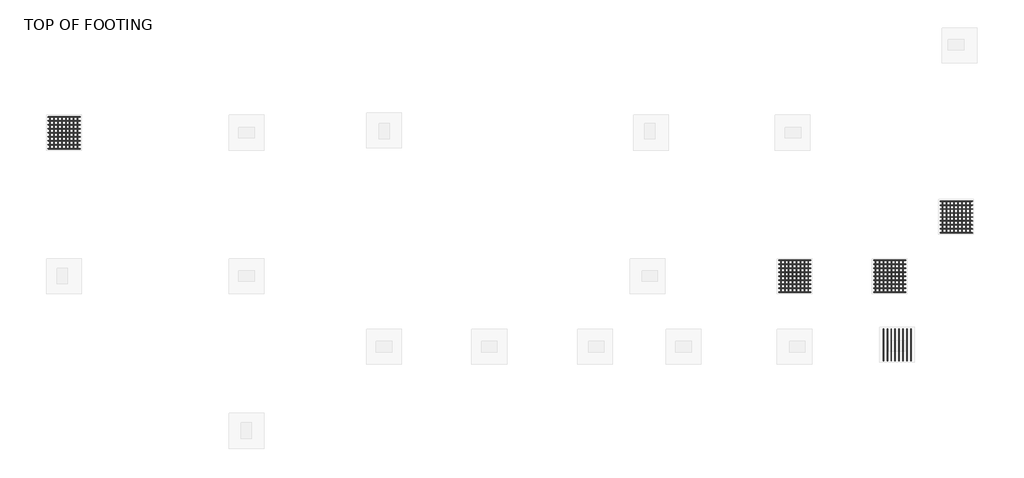
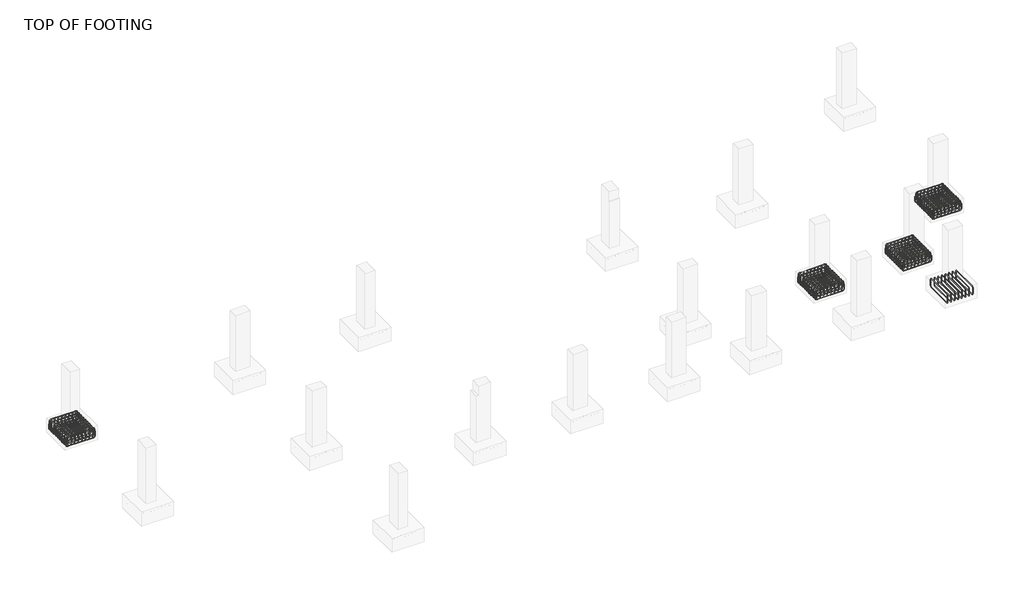
# One storey, part 10 of 20: 18 reinforcing bars.
"""IFC4 building model written with IfcOpenShell, lengths in millimetres."""

from ifc_helpers import new_model, si_unit, point, frame, origin, place, context, project, spatial, polyline, circle_curve, trimmed, segment, composite_curve, source, transform, mapped, element, save
from ifc_brep_helpers import swept_disk

model = new_model("IFC4")

# Units and contexts
model_context = context("Model", 3, world=origin())
ifc_project = project(units=[si_unit("LENGTHUNIT", "METRE", prefix="MILLI")], contexts=[model_context])

# Site, building, storey
site = spatial("IfcSite", under=ifc_project)
building = spatial("IfcBuilding", under=site)
storey = spatial("IfcBuildingStorey", under=building, Name="TOP OF FOOTING", Elevation=-1828.8)

# Reinforcing bars
placement = place(None, origin())
reinforcing_bar_shape = source(origin(), model_context, "Body", "SolidModel", [
    swept_disk(composite_curve([segment(polyline([(14922.7663908, -845.1786071, -2006.6587682), (14922.7663908, -845.1786071, -2153.9587682)]), True, "CONTINUOUS"), segment(trimmed(circle_curve(frame((14876.4163908, -845.1786071, -2153.9587682), z_axis=(0.0, 1.0, 0.0), x_axis=(46.350000000000364, 0.0, 0.0)), 46.35), [point((14922.7663908, -845.1786071, -2153.9587682))], [point((14876.4163908, -845.1786071, -2200.3087682))], True, "CARTESIAN"), True, "CONTINUOUS"), segment(polyline([(14876.4163908, -845.1786071, -2200.3087682), (14061.8163908, -845.1786071, -2200.3087682)]), True, "CONTINUOUS"), segment(trimmed(circle_curve(frame((14061.8163908, -845.1786071, -2153.9587682), z_axis=(0.0, 1.0, 0.0), x_axis=(0.0, 0.0, -46.34999999999991)), 46.35), [point((14061.8163908, -845.1786071, -2200.3087682))], [point((14015.4663908, -845.1786071, -2153.9587682))], True, "CARTESIAN"), True, "CONTINUOUS"), segment(polyline([(14015.4663908, -845.1786071, -2153.9587682), (14015.4663908, -845.1786071, -2006.6587682)]), True, "CONTINUOUS")], self_intersect=False), 6.35),
])
element("IfcReinforcingBar", 1, at=placement, inside=storey, context=model_context, shape_type="MappedRepresentation", body=[
    mapped(reinforcing_bar_shape, transform((0.0, 0.0, 0.0), x_axis=(1.0, 0.0, 0.0), y_axis=(0.0, 1.0, 0.0), z_axis=(0.0, 0.0, 1.0))),
    mapped(reinforcing_bar_shape, transform((0.0, -113.4125, 0.0), x_axis=(1.0, 0.0, 0.0), y_axis=(0.0, 1.0, 0.0), z_axis=(0.0, 0.0, 1.0))),
    mapped(reinforcing_bar_shape, transform((0.0, -226.825, 0.0), x_axis=(1.0, 0.0, 0.0), y_axis=(0.0, 1.0, 0.0), z_axis=(0.0, 0.0, 1.0))),
    mapped(reinforcing_bar_shape, transform((0.0, -340.2375, 0.0), x_axis=(1.0, 0.0, 0.0), y_axis=(0.0, 1.0, 0.0), z_axis=(0.0, 0.0, 1.0))),
    mapped(reinforcing_bar_shape, transform((0.0, -453.65, 0.0), x_axis=(1.0, 0.0, 0.0), y_axis=(0.0, 1.0, 0.0), z_axis=(0.0, 0.0, 1.0))),
    mapped(reinforcing_bar_shape, transform((0.0, -567.0625, 0.0), x_axis=(1.0, 0.0, 0.0), y_axis=(0.0, 1.0, 0.0), z_axis=(0.0, 0.0, 1.0))),
    mapped(reinforcing_bar_shape, transform((0.0, -680.475, 0.0), x_axis=(1.0, 0.0, 0.0), y_axis=(0.0, 1.0, 0.0), z_axis=(0.0, 0.0, 1.0))),
    mapped(reinforcing_bar_shape, transform((0.0, -793.8875, 0.0), x_axis=(1.0, 0.0, 0.0), y_axis=(0.0, 1.0, 0.0), z_axis=(0.0, 0.0, 1.0))),
    mapped(reinforcing_bar_shape, transform((0.0, -907.3, 0.0), x_axis=(1.0, 0.0, 0.0), y_axis=(0.0, 1.0, 0.0), z_axis=(0.0, 0.0, 1.0))),
])
reinforcing_bar_2_shape = source(origin(), model_context, "Body", "SolidModel", [
    swept_disk(composite_curve([segment(polyline([(14034.9405021, -845.1786071, -2068.8), (14034.9405021, -845.1786071, -1921.5)]), True, "CONTINUOUS"), segment(trimmed(circle_curve(frame((14081.2905021, -845.1786071, -1921.5), z_axis=(0.0, 1.0, 0.0), x_axis=(-46.350000000000364, 0.0, 0.0)), 46.35), [point((14034.9405021, -845.1786071, -1921.5))], [point((14081.2905021, -845.1786071, -1875.15))], True, "CARTESIAN"), True, "CONTINUOUS"), segment(polyline([(14081.2905021, -845.1786071, -1875.15), (14850.7539017, -845.1786071, -1875.15)]), True, "CONTINUOUS"), segment(trimmed(circle_curve(frame((14850.7539017, -845.1786071, -1921.5), z_axis=(0.0, 1.0, 0.0), x_axis=(0.0, 0.0, 46.34999999999991)), 46.35), [point((14850.7539017, -845.1786071, -1875.15))], [point((14897.1039017, -845.1786071, -1921.5))], True, "CARTESIAN"), True, "CONTINUOUS"), segment(polyline([(14897.1039017, -845.1786071, -1921.5), (14897.1039017, -845.1786071, -2068.8)]), True, "CONTINUOUS")], self_intersect=False), 6.35),
])
element("IfcReinforcingBar", 2, at=placement, inside=storey, context=model_context, shape_type="MappedRepresentation", body=[
    mapped(reinforcing_bar_2_shape, transform((0.0, 0.0, 0.0), x_axis=(1.0, 0.0, 0.0), y_axis=(0.0, 1.0, 0.0), z_axis=(0.0, 0.0, 1.0))),
    mapped(reinforcing_bar_2_shape, transform((0.0, -113.4125, 0.0), x_axis=(1.0, 0.0, 0.0), y_axis=(0.0, 1.0, 0.0), z_axis=(0.0, 0.0, 1.0))),
    mapped(reinforcing_bar_2_shape, transform((0.0, -226.825, 0.0), x_axis=(1.0, 0.0, 0.0), y_axis=(0.0, 1.0, 0.0), z_axis=(0.0, 0.0, 1.0))),
    mapped(reinforcing_bar_2_shape, transform((0.0, -340.2375, 0.0), x_axis=(1.0, 0.0, 0.0), y_axis=(0.0, 1.0, 0.0), z_axis=(0.0, 0.0, 1.0))),
    mapped(reinforcing_bar_2_shape, transform((0.0, -453.65, 0.0), x_axis=(1.0, 0.0, 0.0), y_axis=(0.0, 1.0, 0.0), z_axis=(0.0, 0.0, 1.0))),
    mapped(reinforcing_bar_2_shape, transform((0.0, -567.0625, 0.0), x_axis=(1.0, 0.0, 0.0), y_axis=(0.0, 1.0, 0.0), z_axis=(0.0, 0.0, 1.0))),
    mapped(reinforcing_bar_2_shape, transform((0.0, -680.475, 0.0), x_axis=(1.0, 0.0, 0.0), y_axis=(0.0, 1.0, 0.0), z_axis=(0.0, 0.0, 1.0))),
    mapped(reinforcing_bar_2_shape, transform((0.0, -793.8875, 0.0), x_axis=(1.0, 0.0, 0.0), y_axis=(0.0, 1.0, 0.0), z_axis=(0.0, 0.0, 1.0))),
    mapped(reinforcing_bar_2_shape, transform((0.0, -907.3, 0.0), x_axis=(1.0, 0.0, 0.0), y_axis=(0.0, 1.0, 0.0), z_axis=(0.0, 0.0, 1.0))),
])
reinforcing_bar_3_shape = source(origin(), model_context, "Body", "SolidModel", [
    swept_disk(composite_curve([segment(polyline([(14851.2694294, -845.1786071, -2086.1951968), (14851.2694294, -845.1786071, -1938.8951968)]), True, "CONTINUOUS"), segment(trimmed(circle_curve(frame((14851.2694294, -891.5286071, -1938.8951968), z_axis=(1.0, 0.0, 0.0), x_axis=(0.0, 46.35000000000002, 0.0)), 46.35), [point((14851.2694294, -845.1786071, -1938.8951968))], [point((14851.2694294, -891.5286071, -1892.5451968))], True, "CARTESIAN"), True, "CONTINUOUS"), segment(polyline([(14851.2694294, -891.5286071, -1892.5451968), (14851.2694294, -1706.1286071, -1892.5451968)]), True, "CONTINUOUS"), segment(trimmed(circle_curve(frame((14851.2694294, -1706.1286071, -1938.8951968), z_axis=(1.0, 0.0, 0.0), x_axis=(0.0, 0.0, 46.34999999999991)), 46.35), [point((14851.2694294, -1706.1286071, -1892.5451968))], [point((14851.2694294, -1752.4786071, -1938.8951968))], True, "CARTESIAN"), True, "CONTINUOUS"), segment(polyline([(14851.2694294, -1752.4786071, -1938.8951968), (14851.2694294, -1752.4786071, -2086.1951968)]), True, "CONTINUOUS")], self_intersect=False), 6.35),
])
element("IfcReinforcingBar", 3, at=placement, inside=storey, context=model_context, shape_type="MappedRepresentation", body=[
    mapped(reinforcing_bar_3_shape, transform((0.0, 0.0, 0.0), x_axis=(1.0, 0.0, 0.0), y_axis=(0.0, 1.0, 0.0), z_axis=(0.0, 0.0, 1.0))),
    mapped(reinforcing_bar_3_shape, transform((-111.2862402, 0.0, 0.0), x_axis=(1.0, 0.0, 0.0), y_axis=(0.0, 1.0, 0.0), z_axis=(0.0, 0.0, 1.0))),
    mapped(reinforcing_bar_3_shape, transform((-222.5724804, 0.0, 0.0), x_axis=(1.0, 0.0, 0.0), y_axis=(0.0, 1.0, 0.0), z_axis=(0.0, 0.0, 1.0))),
    mapped(reinforcing_bar_3_shape, transform((-333.8587205, 0.0, 0.0), x_axis=(1.0, 0.0, 0.0), y_axis=(0.0, 1.0, 0.0), z_axis=(0.0, 0.0, 1.0))),
    mapped(reinforcing_bar_3_shape, transform((-445.1449607, 0.0, 0.0), x_axis=(1.0, 0.0, 0.0), y_axis=(0.0, 1.0, 0.0), z_axis=(0.0, 0.0, 1.0))),
    mapped(reinforcing_bar_3_shape, transform((-556.4312009, 0.0, 0.0), x_axis=(1.0, 0.0, 0.0), y_axis=(0.0, 1.0, 0.0), z_axis=(0.0, 0.0, 1.0))),
    mapped(reinforcing_bar_3_shape, transform((-667.7174411, 0.0, 0.0), x_axis=(1.0, 0.0, 0.0), y_axis=(0.0, 1.0, 0.0), z_axis=(0.0, 0.0, 1.0))),
    mapped(reinforcing_bar_3_shape, transform((-779.0036813, 0.0, 0.0), x_axis=(1.0, 0.0, 0.0), y_axis=(0.0, 1.0, 0.0), z_axis=(0.0, 0.0, 1.0))),
])
reinforcing_bar_4_shape = source(origin(), model_context, "Body", "SolidModel", [
    swept_disk(composite_curve([segment(polyline([(14072.2657481, -845.1786071, -1979.1645013), (14072.2657481, -845.1786071, -2126.4645013)]), True, "CONTINUOUS"), segment(trimmed(circle_curve(frame((14072.2657481, -891.5286071, -2126.4645013), z_axis=(-1.0, 0.0, 0.0), x_axis=(0.0, 46.35000000000002, 0.0)), 46.35), [point((14072.2657481, -845.1786071, -2126.4645013))], [point((14072.2657481, -891.5286071, -2172.8145013))], True, "CARTESIAN"), True, "CONTINUOUS"), segment(polyline([(14072.2657481, -891.5286071, -2172.8145013), (14072.2657481, -1706.1286071, -2172.8145013)]), True, "CONTINUOUS"), segment(trimmed(circle_curve(frame((14072.2657481, -1706.1286071, -2126.4645013), z_axis=(-1.0, 0.0, 0.0), x_axis=(0.0, 0.0, -46.34999999999991)), 46.35), [point((14072.2657481, -1706.1286071, -2172.8145013))], [point((14072.2657481, -1752.4786071, -2126.4645013))], True, "CARTESIAN"), True, "CONTINUOUS"), segment(polyline([(14072.2657481, -1752.4786071, -2126.4645013), (14072.2657481, -1752.4786071, -1979.1645013)]), True, "CONTINUOUS")], self_intersect=False), 6.35),
])
element("IfcReinforcingBar", 4, at=placement, inside=storey, context=model_context, shape_type="MappedRepresentation", body=[
    mapped(reinforcing_bar_4_shape, transform((0.0, 0.0, 0.0), x_axis=(1.0, 0.0, 0.0), y_axis=(0.0, 1.0, 0.0), z_axis=(0.0, 0.0, 1.0))),
    mapped(reinforcing_bar_4_shape, transform((111.2862402, 0.0, 0.0), x_axis=(1.0, 0.0, 0.0), y_axis=(0.0, 1.0, 0.0), z_axis=(0.0, 0.0, 1.0))),
    mapped(reinforcing_bar_4_shape, transform((222.5724804, 0.0, 0.0), x_axis=(1.0, 0.0, 0.0), y_axis=(0.0, 1.0, 0.0), z_axis=(0.0, 0.0, 1.0))),
    mapped(reinforcing_bar_4_shape, transform((333.8587205, 0.0, 0.0), x_axis=(1.0, 0.0, 0.0), y_axis=(0.0, 1.0, 0.0), z_axis=(0.0, 0.0, 1.0))),
    mapped(reinforcing_bar_4_shape, transform((445.1449607, 0.0, 0.0), x_axis=(1.0, 0.0, 0.0), y_axis=(0.0, 1.0, 0.0), z_axis=(0.0, 0.0, 1.0))),
    mapped(reinforcing_bar_4_shape, transform((556.4312009, 0.0, 0.0), x_axis=(1.0, 0.0, 0.0), y_axis=(0.0, 1.0, 0.0), z_axis=(0.0, 0.0, 1.0))),
    mapped(reinforcing_bar_4_shape, transform((667.7174411, 0.0, 0.0), x_axis=(1.0, 0.0, 0.0), y_axis=(0.0, 1.0, 0.0), z_axis=(0.0, 0.0, 1.0))),
    mapped(reinforcing_bar_4_shape, transform((779.0036813, 0.0, 0.0), x_axis=(1.0, 0.0, 0.0), y_axis=(0.0, 1.0, 0.0), z_axis=(0.0, 0.0, 1.0))),
])
reinforcing_bar_5_shape = source(origin(), model_context, "Body", "SolidModel", [
    swept_disk(composite_curve([segment(polyline([(13022.7663908, -2535.8035766, -2006.6587682), (13022.7663908, -2535.8035766, -2153.9587682)]), True, "CONTINUOUS"), segment(trimmed(circle_curve(frame((12976.4163908, -2535.8035766, -2153.9587682), z_axis=(0.0, 1.0, 0.0), x_axis=(46.350000000000364, 0.0, 0.0)), 46.35), [point((13022.7663908, -2535.8035766, -2153.9587682))], [point((12976.4163908, -2535.8035766, -2200.3087682))], True, "CARTESIAN"), True, "CONTINUOUS"), segment(polyline([(12976.4163908, -2535.8035766, -2200.3087682), (12161.8163908, -2535.8035766, -2200.3087682)]), True, "CONTINUOUS"), segment(trimmed(circle_curve(frame((12161.8163908, -2535.8035766, -2153.9587682), z_axis=(0.0, 1.0, 0.0), x_axis=(0.0, 0.0, -46.34999999999991)), 46.35), [point((12161.8163908, -2535.8035766, -2200.3087682))], [point((12115.4663908, -2535.8035766, -2153.9587682))], True, "CARTESIAN"), True, "CONTINUOUS"), segment(polyline([(12115.4663908, -2535.8035766, -2153.9587682), (12115.4663908, -2535.8035766, -2006.6587682)]), True, "CONTINUOUS")], self_intersect=False), 6.35),
])
element("IfcReinforcingBar", 5, at=placement, inside=storey, context=model_context, shape_type="MappedRepresentation", body=[
    mapped(reinforcing_bar_5_shape, transform((0.0, 0.0, 0.0), x_axis=(1.0, 0.0, 0.0), y_axis=(0.0, 1.0, 0.0), z_axis=(0.0, 0.0, 1.0))),
    mapped(reinforcing_bar_5_shape, transform((0.0, -113.4125, 0.0), x_axis=(1.0, 0.0, 0.0), y_axis=(0.0, 1.0, 0.0), z_axis=(0.0, 0.0, 1.0))),
    mapped(reinforcing_bar_5_shape, transform((0.0, -226.825, 0.0), x_axis=(1.0, 0.0, 0.0), y_axis=(0.0, 1.0, 0.0), z_axis=(0.0, 0.0, 1.0))),
    mapped(reinforcing_bar_5_shape, transform((0.0, -340.2375, 0.0), x_axis=(1.0, 0.0, 0.0), y_axis=(0.0, 1.0, 0.0), z_axis=(0.0, 0.0, 1.0))),
    mapped(reinforcing_bar_5_shape, transform((0.0, -453.65, 0.0), x_axis=(1.0, 0.0, 0.0), y_axis=(0.0, 1.0, 0.0), z_axis=(0.0, 0.0, 1.0))),
    mapped(reinforcing_bar_5_shape, transform((0.0, -567.0625, 0.0), x_axis=(1.0, 0.0, 0.0), y_axis=(0.0, 1.0, 0.0), z_axis=(0.0, 0.0, 1.0))),
    mapped(reinforcing_bar_5_shape, transform((0.0, -680.475, 0.0), x_axis=(1.0, 0.0, 0.0), y_axis=(0.0, 1.0, 0.0), z_axis=(0.0, 0.0, 1.0))),
    mapped(reinforcing_bar_5_shape, transform((0.0, -793.8875, 0.0), x_axis=(1.0, 0.0, 0.0), y_axis=(0.0, 1.0, 0.0), z_axis=(0.0, 0.0, 1.0))),
    mapped(reinforcing_bar_5_shape, transform((0.0, -907.3, 0.0), x_axis=(1.0, 0.0, 0.0), y_axis=(0.0, 1.0, 0.0), z_axis=(0.0, 0.0, 1.0))),
])
reinforcing_bar_6_shape = source(origin(), model_context, "Body", "SolidModel", [
    swept_disk(composite_curve([segment(polyline([(12134.9405021, -2535.8035766, -2068.8), (12134.9405021, -2535.8035766, -1921.5)]), True, "CONTINUOUS"), segment(trimmed(circle_curve(frame((12181.2905021, -2535.8035766, -1921.5), z_axis=(0.0, 1.0, 0.0), x_axis=(-46.350000000000364, 0.0, 0.0)), 46.35), [point((12134.9405021, -2535.8035766, -1921.5))], [point((12181.2905021, -2535.8035766, -1875.15))], True, "CARTESIAN"), True, "CONTINUOUS"), segment(polyline([(12181.2905021, -2535.8035766, -1875.15), (12950.7539017, -2535.8035766, -1875.15)]), True, "CONTINUOUS"), segment(trimmed(circle_curve(frame((12950.7539017, -2535.8035766, -1921.5), z_axis=(0.0, 1.0, 0.0), x_axis=(0.0, 0.0, 46.34999999999991)), 46.35), [point((12950.7539017, -2535.8035766, -1875.15))], [point((12997.1039017, -2535.8035766, -1921.5))], True, "CARTESIAN"), True, "CONTINUOUS"), segment(polyline([(12997.1039017, -2535.8035766, -1921.5), (12997.1039017, -2535.8035766, -2068.8)]), True, "CONTINUOUS")], self_intersect=False), 6.35),
])
element("IfcReinforcingBar", 6, at=placement, inside=storey, context=model_context, shape_type="MappedRepresentation", body=[
    mapped(reinforcing_bar_6_shape, transform((0.0, 0.0, 0.0), x_axis=(1.0, 0.0, 0.0), y_axis=(0.0, 1.0, 0.0), z_axis=(0.0, 0.0, 1.0))),
    mapped(reinforcing_bar_6_shape, transform((0.0, -113.4125, 0.0), x_axis=(1.0, 0.0, 0.0), y_axis=(0.0, 1.0, 0.0), z_axis=(0.0, 0.0, 1.0))),
    mapped(reinforcing_bar_6_shape, transform((0.0, -226.825, 0.0), x_axis=(1.0, 0.0, 0.0), y_axis=(0.0, 1.0, 0.0), z_axis=(0.0, 0.0, 1.0))),
    mapped(reinforcing_bar_6_shape, transform((0.0, -340.2375, 0.0), x_axis=(1.0, 0.0, 0.0), y_axis=(0.0, 1.0, 0.0), z_axis=(0.0, 0.0, 1.0))),
    mapped(reinforcing_bar_6_shape, transform((0.0, -453.65, 0.0), x_axis=(1.0, 0.0, 0.0), y_axis=(0.0, 1.0, 0.0), z_axis=(0.0, 0.0, 1.0))),
    mapped(reinforcing_bar_6_shape, transform((0.0, -567.0625, 0.0), x_axis=(1.0, 0.0, 0.0), y_axis=(0.0, 1.0, 0.0), z_axis=(0.0, 0.0, 1.0))),
    mapped(reinforcing_bar_6_shape, transform((0.0, -680.475, 0.0), x_axis=(1.0, 0.0, 0.0), y_axis=(0.0, 1.0, 0.0), z_axis=(0.0, 0.0, 1.0))),
    mapped(reinforcing_bar_6_shape, transform((0.0, -793.8875, 0.0), x_axis=(1.0, 0.0, 0.0), y_axis=(0.0, 1.0, 0.0), z_axis=(0.0, 0.0, 1.0))),
    mapped(reinforcing_bar_6_shape, transform((0.0, -907.3, 0.0), x_axis=(1.0, 0.0, 0.0), y_axis=(0.0, 1.0, 0.0), z_axis=(0.0, 0.0, 1.0))),
])
reinforcing_bar_7_shape = source(origin(), model_context, "Body", "SolidModel", [
    swept_disk(composite_curve([segment(polyline([(12951.2694294, -2535.8035766, -2086.1951968), (12951.2694294, -2535.8035766, -1938.8951968)]), True, "CONTINUOUS"), segment(trimmed(circle_curve(frame((12951.2694294, -2582.1535766, -1938.8951968), z_axis=(1.0, 0.0, 0.0), x_axis=(0.0, 46.350000000000364, 0.0)), 46.35), [point((12951.2694294, -2535.8035766, -1938.8951968))], [point((12951.2694294, -2582.1535766, -1892.5451968))], True, "CARTESIAN"), True, "CONTINUOUS"), segment(polyline([(12951.2694294, -2582.1535766, -1892.5451968), (12951.2694294, -3396.7535766, -1892.5451968)]), True, "CONTINUOUS"), segment(trimmed(circle_curve(frame((12951.2694294, -3396.7535766, -1938.8951968), z_axis=(1.0, 0.0, 0.0), x_axis=(0.0, 0.0, 46.34999999999991)), 46.35), [point((12951.2694294, -3396.7535766, -1892.5451968))], [point((12951.2694294, -3443.1035766, -1938.8951968))], True, "CARTESIAN"), True, "CONTINUOUS"), segment(polyline([(12951.2694294, -3443.1035766, -1938.8951968), (12951.2694294, -3443.1035766, -2086.1951968)]), True, "CONTINUOUS")], self_intersect=False), 6.35),
])
element("IfcReinforcingBar", 7, at=placement, inside=storey, context=model_context, shape_type="MappedRepresentation", body=[
    mapped(reinforcing_bar_7_shape, transform((0.0, 0.0, 0.0), x_axis=(1.0, 0.0, 0.0), y_axis=(0.0, 1.0, 0.0), z_axis=(0.0, 0.0, 1.0))),
    mapped(reinforcing_bar_7_shape, transform((-111.2862402, 0.0, 0.0), x_axis=(1.0, 0.0, 0.0), y_axis=(0.0, 1.0, 0.0), z_axis=(0.0, 0.0, 1.0))),
    mapped(reinforcing_bar_7_shape, transform((-222.5724804, 0.0, 0.0), x_axis=(1.0, 0.0, 0.0), y_axis=(0.0, 1.0, 0.0), z_axis=(0.0, 0.0, 1.0))),
    mapped(reinforcing_bar_7_shape, transform((-333.8587205, 0.0, 0.0), x_axis=(1.0, 0.0, 0.0), y_axis=(0.0, 1.0, 0.0), z_axis=(0.0, 0.0, 1.0))),
    mapped(reinforcing_bar_7_shape, transform((-445.1449607, 0.0, 0.0), x_axis=(1.0, 0.0, 0.0), y_axis=(0.0, 1.0, 0.0), z_axis=(0.0, 0.0, 1.0))),
    mapped(reinforcing_bar_7_shape, transform((-556.4312009, 0.0, 0.0), x_axis=(1.0, 0.0, 0.0), y_axis=(0.0, 1.0, 0.0), z_axis=(0.0, 0.0, 1.0))),
    mapped(reinforcing_bar_7_shape, transform((-667.7174411, 0.0, 0.0), x_axis=(1.0, 0.0, 0.0), y_axis=(0.0, 1.0, 0.0), z_axis=(0.0, 0.0, 1.0))),
    mapped(reinforcing_bar_7_shape, transform((-779.0036813, 0.0, 0.0), x_axis=(1.0, 0.0, 0.0), y_axis=(0.0, 1.0, 0.0), z_axis=(0.0, 0.0, 1.0))),
])
reinforcing_bar_8_shape = source(origin(), model_context, "Body", "SolidModel", [
    swept_disk(composite_curve([segment(polyline([(12172.2657481, -2535.8035766, -1979.1645013), (12172.2657481, -2535.8035766, -2126.4645013)]), True, "CONTINUOUS"), segment(trimmed(circle_curve(frame((12172.2657481, -2582.1535766, -2126.4645013), z_axis=(-1.0, 0.0, 0.0), x_axis=(0.0, 46.350000000000364, 0.0)), 46.35), [point((12172.2657481, -2535.8035766, -2126.4645013))], [point((12172.2657481, -2582.1535766, -2172.8145013))], True, "CARTESIAN"), True, "CONTINUOUS"), segment(polyline([(12172.2657481, -2582.1535766, -2172.8145013), (12172.2657481, -3396.7535766, -2172.8145013)]), True, "CONTINUOUS"), segment(trimmed(circle_curve(frame((12172.2657481, -3396.7535766, -2126.4645013), z_axis=(-1.0, 0.0, 0.0), x_axis=(0.0, 0.0, -46.34999999999991)), 46.35), [point((12172.2657481, -3396.7535766, -2172.8145013))], [point((12172.2657481, -3443.1035766, -2126.4645013))], True, "CARTESIAN"), True, "CONTINUOUS"), segment(polyline([(12172.2657481, -3443.1035766, -2126.4645013), (12172.2657481, -3443.1035766, -1979.1645013)]), True, "CONTINUOUS")], self_intersect=False), 6.35),
])
element("IfcReinforcingBar", 8, at=placement, inside=storey, context=model_context, shape_type="MappedRepresentation", body=[
    mapped(reinforcing_bar_8_shape, transform((0.0, 0.0, 0.0), x_axis=(1.0, 0.0, 0.0), y_axis=(0.0, 1.0, 0.0), z_axis=(0.0, 0.0, 1.0))),
    mapped(reinforcing_bar_8_shape, transform((111.2862402, 0.0, 0.0), x_axis=(1.0, 0.0, 0.0), y_axis=(0.0, 1.0, 0.0), z_axis=(0.0, 0.0, 1.0))),
    mapped(reinforcing_bar_8_shape, transform((222.5724804, 0.0, 0.0), x_axis=(1.0, 0.0, 0.0), y_axis=(0.0, 1.0, 0.0), z_axis=(0.0, 0.0, 1.0))),
    mapped(reinforcing_bar_8_shape, transform((333.8587205, 0.0, 0.0), x_axis=(1.0, 0.0, 0.0), y_axis=(0.0, 1.0, 0.0), z_axis=(0.0, 0.0, 1.0))),
    mapped(reinforcing_bar_8_shape, transform((445.1449607, 0.0, 0.0), x_axis=(1.0, 0.0, 0.0), y_axis=(0.0, 1.0, 0.0), z_axis=(0.0, 0.0, 1.0))),
    mapped(reinforcing_bar_8_shape, transform((556.4312009, 0.0, 0.0), x_axis=(1.0, 0.0, 0.0), y_axis=(0.0, 1.0, 0.0), z_axis=(0.0, 0.0, 1.0))),
    mapped(reinforcing_bar_8_shape, transform((667.7174411, 0.0, 0.0), x_axis=(1.0, 0.0, 0.0), y_axis=(0.0, 1.0, 0.0), z_axis=(0.0, 0.0, 1.0))),
    mapped(reinforcing_bar_8_shape, transform((779.0036813, 0.0, 0.0), x_axis=(1.0, 0.0, 0.0), y_axis=(0.0, 1.0, 0.0), z_axis=(0.0, 0.0, 1.0))),
])
reinforcing_bar_9_shape = source(origin(), model_context, "Body", "SolidModel", [
    swept_disk(composite_curve([segment(polyline([(10322.7663908, -2535.8035766, -2006.6587682), (10322.7663908, -2535.8035766, -2153.9587682)]), True, "CONTINUOUS"), segment(trimmed(circle_curve(frame((10276.4163908, -2535.8035766, -2153.9587682), z_axis=(0.0, 1.0, 0.0), x_axis=(46.350000000000364, 0.0, 0.0)), 46.35), [point((10322.7663908, -2535.8035766, -2153.9587682))], [point((10276.4163908, -2535.8035766, -2200.3087682))], True, "CARTESIAN"), True, "CONTINUOUS"), segment(polyline([(10276.4163908, -2535.8035766, -2200.3087682), (9461.8163908, -2535.8035766, -2200.3087682)]), True, "CONTINUOUS"), segment(trimmed(circle_curve(frame((9461.8163908, -2535.8035766, -2153.9587682), z_axis=(0.0, 1.0, 0.0), x_axis=(0.0, 0.0, -46.34999999999991)), 46.35), [point((9461.8163908, -2535.8035766, -2200.3087682))], [point((9415.4663908, -2535.8035766, -2153.9587682))], True, "CARTESIAN"), True, "CONTINUOUS"), segment(polyline([(9415.4663908, -2535.8035766, -2153.9587682), (9415.4663908, -2535.8035766, -2006.6587682)]), True, "CONTINUOUS")], self_intersect=False), 6.35),
])
element("IfcReinforcingBar", 9, at=placement, inside=storey, context=model_context, shape_type="MappedRepresentation", body=[
    mapped(reinforcing_bar_9_shape, transform((0.0, 0.0, 0.0), x_axis=(1.0, 0.0, 0.0), y_axis=(0.0, 1.0, 0.0), z_axis=(0.0, 0.0, 1.0))),
    mapped(reinforcing_bar_9_shape, transform((0.0, -113.4125, 0.0), x_axis=(1.0, 0.0, 0.0), y_axis=(0.0, 1.0, 0.0), z_axis=(0.0, 0.0, 1.0))),
    mapped(reinforcing_bar_9_shape, transform((0.0, -226.825, 0.0), x_axis=(1.0, 0.0, 0.0), y_axis=(0.0, 1.0, 0.0), z_axis=(0.0, 0.0, 1.0))),
    mapped(reinforcing_bar_9_shape, transform((0.0, -340.2375, 0.0), x_axis=(1.0, 0.0, 0.0), y_axis=(0.0, 1.0, 0.0), z_axis=(0.0, 0.0, 1.0))),
    mapped(reinforcing_bar_9_shape, transform((0.0, -453.65, 0.0), x_axis=(1.0, 0.0, 0.0), y_axis=(0.0, 1.0, 0.0), z_axis=(0.0, 0.0, 1.0))),
    mapped(reinforcing_bar_9_shape, transform((0.0, -567.0625, 0.0), x_axis=(1.0, 0.0, 0.0), y_axis=(0.0, 1.0, 0.0), z_axis=(0.0, 0.0, 1.0))),
    mapped(reinforcing_bar_9_shape, transform((0.0, -680.475, 0.0), x_axis=(1.0, 0.0, 0.0), y_axis=(0.0, 1.0, 0.0), z_axis=(0.0, 0.0, 1.0))),
    mapped(reinforcing_bar_9_shape, transform((0.0, -793.8875, 0.0), x_axis=(1.0, 0.0, 0.0), y_axis=(0.0, 1.0, 0.0), z_axis=(0.0, 0.0, 1.0))),
    mapped(reinforcing_bar_9_shape, transform((0.0, -907.3, 0.0), x_axis=(1.0, 0.0, 0.0), y_axis=(0.0, 1.0, 0.0), z_axis=(0.0, 0.0, 1.0))),
])
reinforcing_bar_10_shape = source(origin(), model_context, "Body", "SolidModel", [
    swept_disk(composite_curve([segment(polyline([(9434.9405021, -2535.8035766, -2068.8), (9434.9405021, -2535.8035766, -1921.5)]), True, "CONTINUOUS"), segment(trimmed(circle_curve(frame((9481.2905021, -2535.8035766, -1921.5), z_axis=(0.0, 1.0, 0.0), x_axis=(-46.350000000000364, 0.0, 0.0)), 46.35), [point((9434.9405021, -2535.8035766, -1921.5))], [point((9481.2905021, -2535.8035766, -1875.15))], True, "CARTESIAN"), True, "CONTINUOUS"), segment(polyline([(9481.2905021, -2535.8035766, -1875.15), (10250.7539017, -2535.8035766, -1875.15)]), True, "CONTINUOUS"), segment(trimmed(circle_curve(frame((10250.7539017, -2535.8035766, -1921.5), z_axis=(0.0, 1.0, 0.0), x_axis=(0.0, 0.0, 46.34999999999991)), 46.35), [point((10250.7539017, -2535.8035766, -1875.15))], [point((10297.1039017, -2535.8035766, -1921.5))], True, "CARTESIAN"), True, "CONTINUOUS"), segment(polyline([(10297.1039017, -2535.8035766, -1921.5), (10297.1039017, -2535.8035766, -2068.8)]), True, "CONTINUOUS")], self_intersect=False), 6.35),
])
element("IfcReinforcingBar", 10, at=placement, inside=storey, context=model_context, shape_type="MappedRepresentation", body=[
    mapped(reinforcing_bar_10_shape, transform((0.0, 0.0, 0.0), x_axis=(1.0, 0.0, 0.0), y_axis=(0.0, 1.0, 0.0), z_axis=(0.0, 0.0, 1.0))),
    mapped(reinforcing_bar_10_shape, transform((0.0, -113.4125, 0.0), x_axis=(1.0, 0.0, 0.0), y_axis=(0.0, 1.0, 0.0), z_axis=(0.0, 0.0, 1.0))),
    mapped(reinforcing_bar_10_shape, transform((0.0, -226.825, 0.0), x_axis=(1.0, 0.0, 0.0), y_axis=(0.0, 1.0, 0.0), z_axis=(0.0, 0.0, 1.0))),
    mapped(reinforcing_bar_10_shape, transform((0.0, -340.2375, 0.0), x_axis=(1.0, 0.0, 0.0), y_axis=(0.0, 1.0, 0.0), z_axis=(0.0, 0.0, 1.0))),
    mapped(reinforcing_bar_10_shape, transform((0.0, -453.65, 0.0), x_axis=(1.0, 0.0, 0.0), y_axis=(0.0, 1.0, 0.0), z_axis=(0.0, 0.0, 1.0))),
    mapped(reinforcing_bar_10_shape, transform((0.0, -567.0625, 0.0), x_axis=(1.0, 0.0, 0.0), y_axis=(0.0, 1.0, 0.0), z_axis=(0.0, 0.0, 1.0))),
    mapped(reinforcing_bar_10_shape, transform((0.0, -680.475, 0.0), x_axis=(1.0, 0.0, 0.0), y_axis=(0.0, 1.0, 0.0), z_axis=(0.0, 0.0, 1.0))),
    mapped(reinforcing_bar_10_shape, transform((0.0, -793.8875, 0.0), x_axis=(1.0, 0.0, 0.0), y_axis=(0.0, 1.0, 0.0), z_axis=(0.0, 0.0, 1.0))),
    mapped(reinforcing_bar_10_shape, transform((0.0, -907.3, 0.0), x_axis=(1.0, 0.0, 0.0), y_axis=(0.0, 1.0, 0.0), z_axis=(0.0, 0.0, 1.0))),
])
reinforcing_bar_11_shape = source(origin(), model_context, "Body", "SolidModel", [
    swept_disk(composite_curve([segment(polyline([(10251.2694294, -2535.8035766, -2086.1951968), (10251.2694294, -2535.8035766, -1938.8951968)]), True, "CONTINUOUS"), segment(trimmed(circle_curve(frame((10251.2694294, -2582.1535766, -1938.8951968), z_axis=(1.0, 0.0, 0.0), x_axis=(0.0, 46.350000000000364, 0.0)), 46.35), [point((10251.2694294, -2535.8035766, -1938.8951968))], [point((10251.2694294, -2582.1535766, -1892.5451968))], True, "CARTESIAN"), True, "CONTINUOUS"), segment(polyline([(10251.2694294, -2582.1535766, -1892.5451968), (10251.2694294, -3396.7535766, -1892.5451968)]), True, "CONTINUOUS"), segment(trimmed(circle_curve(frame((10251.2694294, -3396.7535766, -1938.8951968), z_axis=(1.0, 0.0, 0.0), x_axis=(0.0, 0.0, 46.34999999999991)), 46.35), [point((10251.2694294, -3396.7535766, -1892.5451968))], [point((10251.2694294, -3443.1035766, -1938.8951968))], True, "CARTESIAN"), True, "CONTINUOUS"), segment(polyline([(10251.2694294, -3443.1035766, -1938.8951968), (10251.2694294, -3443.1035766, -2086.1951968)]), True, "CONTINUOUS")], self_intersect=False), 6.35),
])
element("IfcReinforcingBar", 11, at=placement, inside=storey, context=model_context, shape_type="MappedRepresentation", body=[
    mapped(reinforcing_bar_11_shape, transform((0.0, 0.0, 0.0), x_axis=(1.0, 0.0, 0.0), y_axis=(0.0, 1.0, 0.0), z_axis=(0.0, 0.0, 1.0))),
    mapped(reinforcing_bar_11_shape, transform((-111.2862402, 0.0, 0.0), x_axis=(1.0, 0.0, 0.0), y_axis=(0.0, 1.0, 0.0), z_axis=(0.0, 0.0, 1.0))),
    mapped(reinforcing_bar_11_shape, transform((-222.5724804, 0.0, 0.0), x_axis=(1.0, 0.0, 0.0), y_axis=(0.0, 1.0, 0.0), z_axis=(0.0, 0.0, 1.0))),
    mapped(reinforcing_bar_11_shape, transform((-333.8587205, 0.0, 0.0), x_axis=(1.0, 0.0, 0.0), y_axis=(0.0, 1.0, 0.0), z_axis=(0.0, 0.0, 1.0))),
    mapped(reinforcing_bar_11_shape, transform((-445.1449607, 0.0, 0.0), x_axis=(1.0, 0.0, 0.0), y_axis=(0.0, 1.0, 0.0), z_axis=(0.0, 0.0, 1.0))),
    mapped(reinforcing_bar_11_shape, transform((-556.4312009, 0.0, 0.0), x_axis=(1.0, 0.0, 0.0), y_axis=(0.0, 1.0, 0.0), z_axis=(0.0, 0.0, 1.0))),
    mapped(reinforcing_bar_11_shape, transform((-667.7174411, 0.0, 0.0), x_axis=(1.0, 0.0, 0.0), y_axis=(0.0, 1.0, 0.0), z_axis=(0.0, 0.0, 1.0))),
    mapped(reinforcing_bar_11_shape, transform((-779.0036813, 0.0, 0.0), x_axis=(1.0, 0.0, 0.0), y_axis=(0.0, 1.0, 0.0), z_axis=(0.0, 0.0, 1.0))),
])
reinforcing_bar_12_shape = source(origin(), model_context, "Body", "SolidModel", [
    swept_disk(composite_curve([segment(polyline([(9472.2657481, -2535.8035766, -1979.1645013), (9472.2657481, -2535.8035766, -2126.4645013)]), True, "CONTINUOUS"), segment(trimmed(circle_curve(frame((9472.2657481, -2582.1535766, -2126.4645013), z_axis=(-1.0, 0.0, 0.0), x_axis=(0.0, 46.350000000000364, 0.0)), 46.35), [point((9472.2657481, -2535.8035766, -2126.4645013))], [point((9472.2657481, -2582.1535766, -2172.8145013))], True, "CARTESIAN"), True, "CONTINUOUS"), segment(polyline([(9472.2657481, -2582.1535766, -2172.8145013), (9472.2657481, -3396.7535766, -2172.8145013)]), True, "CONTINUOUS"), segment(trimmed(circle_curve(frame((9472.2657481, -3396.7535766, -2126.4645013), z_axis=(-1.0, 0.0, 0.0), x_axis=(0.0, 0.0, -46.34999999999991)), 46.35), [point((9472.2657481, -3396.7535766, -2172.8145013))], [point((9472.2657481, -3443.1035766, -2126.4645013))], True, "CARTESIAN"), True, "CONTINUOUS"), segment(polyline([(9472.2657481, -3443.1035766, -2126.4645013), (9472.2657481, -3443.1035766, -1979.1645013)]), True, "CONTINUOUS")], self_intersect=False), 6.35),
])
element("IfcReinforcingBar", 12, at=placement, inside=storey, context=model_context, shape_type="MappedRepresentation", body=[
    mapped(reinforcing_bar_12_shape, transform((0.0, 0.0, 0.0), x_axis=(1.0, 0.0, 0.0), y_axis=(0.0, 1.0, 0.0), z_axis=(0.0, 0.0, 1.0))),
    mapped(reinforcing_bar_12_shape, transform((111.2862402, 0.0, 0.0), x_axis=(1.0, 0.0, 0.0), y_axis=(0.0, 1.0, 0.0), z_axis=(0.0, 0.0, 1.0))),
    mapped(reinforcing_bar_12_shape, transform((222.5724804, 0.0, 0.0), x_axis=(1.0, 0.0, 0.0), y_axis=(0.0, 1.0, 0.0), z_axis=(0.0, 0.0, 1.0))),
    mapped(reinforcing_bar_12_shape, transform((333.8587205, 0.0, 0.0), x_axis=(1.0, 0.0, 0.0), y_axis=(0.0, 1.0, 0.0), z_axis=(0.0, 0.0, 1.0))),
    mapped(reinforcing_bar_12_shape, transform((445.1449607, 0.0, 0.0), x_axis=(1.0, 0.0, 0.0), y_axis=(0.0, 1.0, 0.0), z_axis=(0.0, 0.0, 1.0))),
    mapped(reinforcing_bar_12_shape, transform((556.4312009, 0.0, 0.0), x_axis=(1.0, 0.0, 0.0), y_axis=(0.0, 1.0, 0.0), z_axis=(0.0, 0.0, 1.0))),
    mapped(reinforcing_bar_12_shape, transform((667.7174411, 0.0, 0.0), x_axis=(1.0, 0.0, 0.0), y_axis=(0.0, 1.0, 0.0), z_axis=(0.0, 0.0, 1.0))),
    mapped(reinforcing_bar_12_shape, transform((779.0036813, 0.0, 0.0), x_axis=(1.0, 0.0, 0.0), y_axis=(0.0, 1.0, 0.0), z_axis=(0.0, 0.0, 1.0))),
])
reinforcing_bar_13_shape = source(origin(), model_context, "Body", "SolidModel", [
    swept_disk(composite_curve([segment(polyline([(13171.2694294, -4487.9729916, -2086.1951968), (13171.2694294, -4487.9729916, -1938.8951968)]), True, "CONTINUOUS"), segment(trimmed(circle_curve(frame((13171.2694294, -4534.3229916, -1938.8951968), z_axis=(1.0, 0.0, 0.0), x_axis=(0.0, 46.350000000000364, 0.0)), 46.35), [point((13171.2694294, -4487.9729916, -1938.8951968))], [point((13171.2694294, -4534.3229916, -1892.5451968))], True, "CARTESIAN"), True, "CONTINUOUS"), segment(polyline([(13171.2694294, -4534.3229916, -1892.5451968), (13171.2694294, -5348.9229916, -1892.5451968)]), True, "CONTINUOUS"), segment(trimmed(circle_curve(frame((13171.2694294, -5348.9229916, -1938.8951968), z_axis=(1.0, 0.0, 0.0), x_axis=(0.0, 0.0, 46.34999999999991)), 46.35), [point((13171.2694294, -5348.9229916, -1892.5451968))], [point((13171.2694294, -5395.2729916, -1938.8951968))], True, "CARTESIAN"), True, "CONTINUOUS"), segment(polyline([(13171.2694294, -5395.2729916, -1938.8951968), (13171.2694294, -5395.2729916, -2086.1951968)]), True, "CONTINUOUS")], self_intersect=False), 6.35),
])
element("IfcReinforcingBar", 13, at=placement, inside=storey, context=model_context, shape_type="MappedRepresentation", body=[
    mapped(reinforcing_bar_13_shape, transform((0.0, 0.0, 0.0), x_axis=(1.0, 0.0, 0.0), y_axis=(0.0, 1.0, 0.0), z_axis=(0.0, 0.0, 1.0))),
    mapped(reinforcing_bar_13_shape, transform((-111.2862402, 0.0, 0.0), x_axis=(1.0, 0.0, 0.0), y_axis=(0.0, 1.0, 0.0), z_axis=(0.0, 0.0, 1.0))),
    mapped(reinforcing_bar_13_shape, transform((-222.5724804, 0.0, 0.0), x_axis=(1.0, 0.0, 0.0), y_axis=(0.0, 1.0, 0.0), z_axis=(0.0, 0.0, 1.0))),
    mapped(reinforcing_bar_13_shape, transform((-333.8587205, 0.0, 0.0), x_axis=(1.0, 0.0, 0.0), y_axis=(0.0, 1.0, 0.0), z_axis=(0.0, 0.0, 1.0))),
    mapped(reinforcing_bar_13_shape, transform((-445.1449607, 0.0, 0.0), x_axis=(1.0, 0.0, 0.0), y_axis=(0.0, 1.0, 0.0), z_axis=(0.0, 0.0, 1.0))),
    mapped(reinforcing_bar_13_shape, transform((-556.4312009, 0.0, 0.0), x_axis=(1.0, 0.0, 0.0), y_axis=(0.0, 1.0, 0.0), z_axis=(0.0, 0.0, 1.0))),
    mapped(reinforcing_bar_13_shape, transform((-667.7174411, 0.0, 0.0), x_axis=(1.0, 0.0, 0.0), y_axis=(0.0, 1.0, 0.0), z_axis=(0.0, 0.0, 1.0))),
    mapped(reinforcing_bar_13_shape, transform((-779.0036813, 0.0, 0.0), x_axis=(1.0, 0.0, 0.0), y_axis=(0.0, 1.0, 0.0), z_axis=(0.0, 0.0, 1.0))),
])
reinforcing_bar_14_shape = source(origin(), model_context, "Body", "SolidModel", [
    swept_disk(composite_curve([segment(polyline([(12392.2657481, -4487.9729916, -1979.1645013), (12392.2657481, -4487.9729916, -2126.4645013)]), True, "CONTINUOUS"), segment(trimmed(circle_curve(frame((12392.2657481, -4534.3229916, -2126.4645013), z_axis=(-1.0, 0.0, 0.0), x_axis=(0.0, 46.350000000000364, 0.0)), 46.35), [point((12392.2657481, -4487.9729916, -2126.4645013))], [point((12392.2657481, -4534.3229916, -2172.8145013))], True, "CARTESIAN"), True, "CONTINUOUS"), segment(polyline([(12392.2657481, -4534.3229916, -2172.8145013), (12392.2657481, -5348.9229916, -2172.8145013)]), True, "CONTINUOUS"), segment(trimmed(circle_curve(frame((12392.2657481, -5348.9229916, -2126.4645013), z_axis=(-1.0, 0.0, 0.0), x_axis=(0.0, 0.0, -46.34999999999991)), 46.35), [point((12392.2657481, -5348.9229916, -2172.8145013))], [point((12392.2657481, -5395.2729916, -2126.4645013))], True, "CARTESIAN"), True, "CONTINUOUS"), segment(polyline([(12392.2657481, -5395.2729916, -2126.4645013), (12392.2657481, -5395.2729916, -1979.1645013)]), True, "CONTINUOUS")], self_intersect=False), 6.35),
])
element("IfcReinforcingBar", 14, at=placement, inside=storey, context=model_context, shape_type="MappedRepresentation", body=[
    mapped(reinforcing_bar_14_shape, transform((0.0, 0.0, 0.0), x_axis=(1.0, 0.0, 0.0), y_axis=(0.0, 1.0, 0.0), z_axis=(0.0, 0.0, 1.0))),
    mapped(reinforcing_bar_14_shape, transform((111.2862402, 0.0, 0.0), x_axis=(1.0, 0.0, 0.0), y_axis=(0.0, 1.0, 0.0), z_axis=(0.0, 0.0, 1.0))),
    mapped(reinforcing_bar_14_shape, transform((222.5724804, 0.0, 0.0), x_axis=(1.0, 0.0, 0.0), y_axis=(0.0, 1.0, 0.0), z_axis=(0.0, 0.0, 1.0))),
    mapped(reinforcing_bar_14_shape, transform((333.8587205, 0.0, 0.0), x_axis=(1.0, 0.0, 0.0), y_axis=(0.0, 1.0, 0.0), z_axis=(0.0, 0.0, 1.0))),
    mapped(reinforcing_bar_14_shape, transform((445.1449607, 0.0, 0.0), x_axis=(1.0, 0.0, 0.0), y_axis=(0.0, 1.0, 0.0), z_axis=(0.0, 0.0, 1.0))),
    mapped(reinforcing_bar_14_shape, transform((556.4312009, 0.0, 0.0), x_axis=(1.0, 0.0, 0.0), y_axis=(0.0, 1.0, 0.0), z_axis=(0.0, 0.0, 1.0))),
    mapped(reinforcing_bar_14_shape, transform((667.7174411, 0.0, 0.0), x_axis=(1.0, 0.0, 0.0), y_axis=(0.0, 1.0, 0.0), z_axis=(0.0, 0.0, 1.0))),
    mapped(reinforcing_bar_14_shape, transform((779.0036813, 0.0, 0.0), x_axis=(1.0, 0.0, 0.0), y_axis=(0.0, 1.0, 0.0), z_axis=(0.0, 0.0, 1.0))),
])
reinforcing_bar_15_shape = source(origin(), model_context, "Body", "SolidModel", [
    swept_disk(composite_curve([segment(polyline([(-10485.1605653, 1554.8213929, -2006.6587682), (-10485.1605653, 1554.8213929, -2153.9587682)]), True, "CONTINUOUS"), segment(trimmed(circle_curve(frame((-10531.5105653, 1554.8213929, -2153.9587682), z_axis=(0.0, 1.0, 0.0), x_axis=(46.349999999998545, 0.0, 0.0)), 46.35), [point((-10485.1605653, 1554.8213929, -2153.9587682))], [point((-10531.5105653, 1554.8213929, -2200.3087682))], True, "CARTESIAN"), True, "CONTINUOUS"), segment(polyline([(-10531.5105653, 1554.8213929, -2200.3087682), (-11346.1105653, 1554.8213929, -2200.3087682)]), True, "CONTINUOUS"), segment(trimmed(circle_curve(frame((-11346.1105653, 1554.8213929, -2153.9587682), z_axis=(0.0, 1.0, 0.0), x_axis=(0.0, 0.0, -46.34999999999991)), 46.35), [point((-11346.1105653, 1554.8213929, -2200.3087682))], [point((-11392.4605653, 1554.8213929, -2153.9587682))], True, "CARTESIAN"), True, "CONTINUOUS"), segment(polyline([(-11392.4605653, 1554.8213929, -2153.9587682), (-11392.4605653, 1554.8213929, -2006.6587682)]), True, "CONTINUOUS")], self_intersect=False), 6.35),
])
element("IfcReinforcingBar", 15, at=placement, inside=storey, context=model_context, shape_type="MappedRepresentation", body=[
    mapped(reinforcing_bar_15_shape, transform((0.0, 0.0, 0.0), x_axis=(1.0, 0.0, 0.0), y_axis=(0.0, 1.0, 0.0), z_axis=(0.0, 0.0, 1.0))),
    mapped(reinforcing_bar_15_shape, transform((0.0, -113.4125, 0.0), x_axis=(1.0, 0.0, 0.0), y_axis=(0.0, 1.0, 0.0), z_axis=(0.0, 0.0, 1.0))),
    mapped(reinforcing_bar_15_shape, transform((0.0, -226.825, 0.0), x_axis=(1.0, 0.0, 0.0), y_axis=(0.0, 1.0, 0.0), z_axis=(0.0, 0.0, 1.0))),
    mapped(reinforcing_bar_15_shape, transform((0.0, -340.2375, 0.0), x_axis=(1.0, 0.0, 0.0), y_axis=(0.0, 1.0, 0.0), z_axis=(0.0, 0.0, 1.0))),
    mapped(reinforcing_bar_15_shape, transform((0.0, -453.65, 0.0), x_axis=(1.0, 0.0, 0.0), y_axis=(0.0, 1.0, 0.0), z_axis=(0.0, 0.0, 1.0))),
    mapped(reinforcing_bar_15_shape, transform((0.0, -567.0625, 0.0), x_axis=(1.0, 0.0, 0.0), y_axis=(0.0, 1.0, 0.0), z_axis=(0.0, 0.0, 1.0))),
    mapped(reinforcing_bar_15_shape, transform((0.0, -680.475, 0.0), x_axis=(1.0, 0.0, 0.0), y_axis=(0.0, 1.0, 0.0), z_axis=(0.0, 0.0, 1.0))),
    mapped(reinforcing_bar_15_shape, transform((0.0, -793.8875, 0.0), x_axis=(1.0, 0.0, 0.0), y_axis=(0.0, 1.0, 0.0), z_axis=(0.0, 0.0, 1.0))),
    mapped(reinforcing_bar_15_shape, transform((0.0, -907.3, 0.0), x_axis=(1.0, 0.0, 0.0), y_axis=(0.0, 1.0, 0.0), z_axis=(0.0, 0.0, 1.0))),
])
reinforcing_bar_16_shape = source(origin(), model_context, "Body", "SolidModel", [
    swept_disk(composite_curve([segment(polyline([(-11372.986454, 1554.8213929, -2068.8), (-11372.986454, 1554.8213929, -1921.5)]), True, "CONTINUOUS"), segment(trimmed(circle_curve(frame((-11326.636454, 1554.8213929, -1921.5), z_axis=(0.0, 1.0, 0.0), x_axis=(-46.350000000000364, 0.0, 0.0)), 46.35), [point((-11372.986454, 1554.8213929, -1921.5))], [point((-11326.636454, 1554.8213929, -1875.15))], True, "CARTESIAN"), True, "CONTINUOUS"), segment(polyline([(-11326.636454, 1554.8213929, -1875.15), (-10557.1730543, 1554.8213929, -1875.15)]), True, "CONTINUOUS"), segment(trimmed(circle_curve(frame((-10557.1730543, 1554.8213929, -1921.5), z_axis=(0.0, 1.0, 0.0), x_axis=(0.0, 0.0, 46.34999999999991)), 46.35), [point((-10557.1730543, 1554.8213929, -1875.15))], [point((-10510.8230543, 1554.8213929, -1921.5))], True, "CARTESIAN"), True, "CONTINUOUS"), segment(polyline([(-10510.8230543, 1554.8213929, -1921.5), (-10510.8230543, 1554.8213929, -2068.8)]), True, "CONTINUOUS")], self_intersect=False), 6.35),
])
element("IfcReinforcingBar", 16, at=placement, inside=storey, context=model_context, shape_type="MappedRepresentation", body=[
    mapped(reinforcing_bar_16_shape, transform((0.0, 0.0, 0.0), x_axis=(1.0, 0.0, 0.0), y_axis=(0.0, 1.0, 0.0), z_axis=(0.0, 0.0, 1.0))),
    mapped(reinforcing_bar_16_shape, transform((0.0, -113.4125, 0.0), x_axis=(1.0, 0.0, 0.0), y_axis=(0.0, 1.0, 0.0), z_axis=(0.0, 0.0, 1.0))),
    mapped(reinforcing_bar_16_shape, transform((0.0, -226.825, 0.0), x_axis=(1.0, 0.0, 0.0), y_axis=(0.0, 1.0, 0.0), z_axis=(0.0, 0.0, 1.0))),
    mapped(reinforcing_bar_16_shape, transform((0.0, -340.2375, 0.0), x_axis=(1.0, 0.0, 0.0), y_axis=(0.0, 1.0, 0.0), z_axis=(0.0, 0.0, 1.0))),
    mapped(reinforcing_bar_16_shape, transform((0.0, -453.65, 0.0), x_axis=(1.0, 0.0, 0.0), y_axis=(0.0, 1.0, 0.0), z_axis=(0.0, 0.0, 1.0))),
    mapped(reinforcing_bar_16_shape, transform((0.0, -567.0625, 0.0), x_axis=(1.0, 0.0, 0.0), y_axis=(0.0, 1.0, 0.0), z_axis=(0.0, 0.0, 1.0))),
    mapped(reinforcing_bar_16_shape, transform((0.0, -680.475, 0.0), x_axis=(1.0, 0.0, 0.0), y_axis=(0.0, 1.0, 0.0), z_axis=(0.0, 0.0, 1.0))),
    mapped(reinforcing_bar_16_shape, transform((0.0, -793.8875, 0.0), x_axis=(1.0, 0.0, 0.0), y_axis=(0.0, 1.0, 0.0), z_axis=(0.0, 0.0, 1.0))),
    mapped(reinforcing_bar_16_shape, transform((0.0, -907.3, 0.0), x_axis=(1.0, 0.0, 0.0), y_axis=(0.0, 1.0, 0.0), z_axis=(0.0, 0.0, 1.0))),
])
reinforcing_bar_17_shape = source(origin(), model_context, "Body", "SolidModel", [
    swept_disk(composite_curve([segment(polyline([(-10556.6575267, 1554.8213929, -2086.1951968), (-10556.6575267, 1554.8213929, -1938.8951968)]), True, "CONTINUOUS"), segment(trimmed(circle_curve(frame((-10556.6575267, 1508.4713929, -1938.8951968), z_axis=(1.0, 0.0, 0.0), x_axis=(0.0, 46.350000000000136, 0.0)), 46.35), [point((-10556.6575267, 1554.8213929, -1938.8951968))], [point((-10556.6575267, 1508.4713929, -1892.5451968))], True, "CARTESIAN"), True, "CONTINUOUS"), segment(polyline([(-10556.6575267, 1508.4713929, -1892.5451968), (-10556.6575267, 693.8713929, -1892.5451968)]), True, "CONTINUOUS"), segment(trimmed(circle_curve(frame((-10556.6575267, 693.8713929, -1938.8951968), z_axis=(1.0, 0.0, 0.0), x_axis=(0.0, 0.0, 46.34999999999991)), 46.35), [point((-10556.6575267, 693.8713929, -1892.5451968))], [point((-10556.6575267, 647.5213929, -1938.8951968))], True, "CARTESIAN"), True, "CONTINUOUS"), segment(polyline([(-10556.6575267, 647.5213929, -1938.8951968), (-10556.6575267, 647.5213929, -2086.1951968)]), True, "CONTINUOUS")], self_intersect=False), 6.35),
])
element("IfcReinforcingBar", 17, at=placement, inside=storey, context=model_context, shape_type="MappedRepresentation", body=[
    mapped(reinforcing_bar_17_shape, transform((0.0, 0.0, 0.0), x_axis=(1.0, 0.0, 0.0), y_axis=(0.0, 1.0, 0.0), z_axis=(0.0, 0.0, 1.0))),
    mapped(reinforcing_bar_17_shape, transform((-111.2862402, 0.0, 0.0), x_axis=(1.0, 0.0, 0.0), y_axis=(0.0, 1.0, 0.0), z_axis=(0.0, 0.0, 1.0))),
    mapped(reinforcing_bar_17_shape, transform((-222.5724804, 0.0, 0.0), x_axis=(1.0, 0.0, 0.0), y_axis=(0.0, 1.0, 0.0), z_axis=(0.0, 0.0, 1.0))),
    mapped(reinforcing_bar_17_shape, transform((-333.8587205, 0.0, 0.0), x_axis=(1.0, 0.0, 0.0), y_axis=(0.0, 1.0, 0.0), z_axis=(0.0, 0.0, 1.0))),
    mapped(reinforcing_bar_17_shape, transform((-445.1449607, 0.0, 0.0), x_axis=(1.0, 0.0, 0.0), y_axis=(0.0, 1.0, 0.0), z_axis=(0.0, 0.0, 1.0))),
    mapped(reinforcing_bar_17_shape, transform((-556.4312009, 0.0, 0.0), x_axis=(1.0, 0.0, 0.0), y_axis=(0.0, 1.0, 0.0), z_axis=(0.0, 0.0, 1.0))),
    mapped(reinforcing_bar_17_shape, transform((-667.7174411, 0.0, 0.0), x_axis=(1.0, 0.0, 0.0), y_axis=(0.0, 1.0, 0.0), z_axis=(0.0, 0.0, 1.0))),
    mapped(reinforcing_bar_17_shape, transform((-779.0036813, 0.0, 0.0), x_axis=(1.0, 0.0, 0.0), y_axis=(0.0, 1.0, 0.0), z_axis=(0.0, 0.0, 1.0))),
])
reinforcing_bar_18_shape = source(origin(), model_context, "Body", "SolidModel", [
    swept_disk(composite_curve([segment(polyline([(-11335.661208, 1554.8213929, -1979.1645013), (-11335.661208, 1554.8213929, -2126.4645013)]), True, "CONTINUOUS"), segment(trimmed(circle_curve(frame((-11335.661208, 1508.4713929, -2126.4645013), z_axis=(-1.0, 0.0, 0.0), x_axis=(0.0, 46.350000000000136, 0.0)), 46.35), [point((-11335.661208, 1554.8213929, -2126.4645013))], [point((-11335.661208, 1508.4713929, -2172.8145013))], True, "CARTESIAN"), True, "CONTINUOUS"), segment(polyline([(-11335.661208, 1508.4713929, -2172.8145013), (-11335.661208, 693.8713929, -2172.8145013)]), True, "CONTINUOUS"), segment(trimmed(circle_curve(frame((-11335.661208, 693.8713929, -2126.4645013), z_axis=(-1.0, 0.0, 0.0), x_axis=(0.0, 0.0, -46.34999999999991)), 46.35), [point((-11335.661208, 693.8713929, -2172.8145013))], [point((-11335.661208, 647.5213929, -2126.4645013))], True, "CARTESIAN"), True, "CONTINUOUS"), segment(polyline([(-11335.661208, 647.5213929, -2126.4645013), (-11335.661208, 647.5213929, -1979.1645013)]), True, "CONTINUOUS")], self_intersect=False), 6.35),
])
element("IfcReinforcingBar", 18, at=placement, inside=storey, context=model_context, shape_type="MappedRepresentation", body=[
    mapped(reinforcing_bar_18_shape, transform((0.0, 0.0, 0.0), x_axis=(1.0, 0.0, 0.0), y_axis=(0.0, 1.0, 0.0), z_axis=(0.0, 0.0, 1.0))),
    mapped(reinforcing_bar_18_shape, transform((111.2862402, 0.0, 0.0), x_axis=(1.0, 0.0, 0.0), y_axis=(0.0, 1.0, 0.0), z_axis=(0.0, 0.0, 1.0))),
    mapped(reinforcing_bar_18_shape, transform((222.5724804, 0.0, 0.0), x_axis=(1.0, 0.0, 0.0), y_axis=(0.0, 1.0, 0.0), z_axis=(0.0, 0.0, 1.0))),
    mapped(reinforcing_bar_18_shape, transform((333.8587205, 0.0, 0.0), x_axis=(1.0, 0.0, 0.0), y_axis=(0.0, 1.0, 0.0), z_axis=(0.0, 0.0, 1.0))),
    mapped(reinforcing_bar_18_shape, transform((445.1449607, 0.0, 0.0), x_axis=(1.0, 0.0, 0.0), y_axis=(0.0, 1.0, 0.0), z_axis=(0.0, 0.0, 1.0))),
    mapped(reinforcing_bar_18_shape, transform((556.4312009, 0.0, 0.0), x_axis=(1.0, 0.0, 0.0), y_axis=(0.0, 1.0, 0.0), z_axis=(0.0, 0.0, 1.0))),
    mapped(reinforcing_bar_18_shape, transform((667.7174411, 0.0, 0.0), x_axis=(1.0, 0.0, 0.0), y_axis=(0.0, 1.0, 0.0), z_axis=(0.0, 0.0, 1.0))),
    mapped(reinforcing_bar_18_shape, transform((779.0036813, 0.0, 0.0), x_axis=(1.0, 0.0, 0.0), y_axis=(0.0, 1.0, 0.0), z_axis=(0.0, 0.0, 1.0))),
])

save(model, "model.ifc")

# Revit data of these elements
# Elements 1, 2, 3, 4, 5, 6, 7, 8, 9, 10, 11, 12, 13, 14, 15, 16, 17, 18 (IfcReinforcingBar)
#   Phase Created = New Construction
